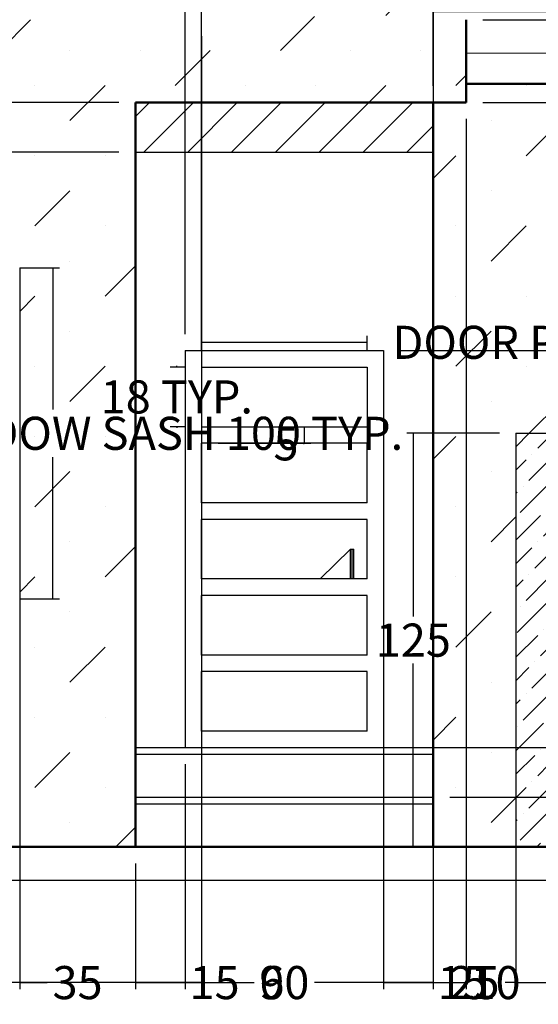
# Model space of a CAD drawing. Units: millimetres. Extents: x 301 to 1039, y -12 to 673.
# Tile 2 of 6: x 579 to 736, y -12 to 285. Entities that reach past the tile are written whole.
import ezdxf

# ---------------------------------------------------------------- set-up
doc = ezdxf.new("R2010")
doc.units = ezdxf.units.MM
doc.header["$MEASUREMENT"] = 0
for name, color, linetype, lineweight in [('A-ANNO-DIMS', 2, 'Continuous', 18), ('A-DOOR', 4, 'Continuous', 25), ('A-ELEV', 8, 'Continuous', 25), ('A-FLOR-STRS', 3, 'Continuous', 25), ('A-WALL', 7, 'Continuous', 50), ('A-WALL-PATT', 9, 'Continuous', 13)]:
    doc.layers.add(name, color=color, linetype=linetype, lineweight=lineweight)
doc.styles.get("Standard").update_dxf_attribs({"font": 'arial.ttf'})
doc.dimstyles.get("Standard").update_dxf_attribs({"dimtxt": 10, "dimasz": 0.18, "dimexe": 2, "dimexo": 5, "dimgap": 2, "dimtad": 0, "dimtih": 1, "dimtoh": 1, "dimdec": 0, "dimzin": 0, "dimdsep": 46, "dimtxsty": 'Standard', "dimcen": 0.09, "dimadec": 0, "dimazin": 0, "dimtfac": 1, "dimtdec": 0, "dimtofl": 0, "dimtmove": 0, "dimatfit": 3, "dimfxl": 1, "dimtolj": 1, "dimtzin": 0, "dimarcsym": 0})

# ---------------------------------------------------------------- blocks, each defined once
blk = doc.blocks.new('DOOR-PANEL')
for p, q in [((0, 18), (50, 18)), ((0, 18), (0, 0)), ((50, 18), (50, 0)), ((0, 0), (50, 0))]:
    blk.add_line(p, q)
blk = doc.blocks.new('*D10')
at = {"layer": 'A-ANNO-DIMS', "color": 0, "lineweight": -2, "transparency": 16777216}
for p, q in [((633.79, 185.09), (633.79, 189.59)), ((633.97, 187.59), (683.61, 187.59)), ((683.79, 185.09), (683.79, 189.59)), ((683.79, 187.59), (683.97, 187.59))]:
    blk.add_line(p, q, dxfattribs=at)
at = {"layer": 'A-ANNO-DIMS', "color": 0, "transparency": 16777216}
for points in [[(633.97, 187.62), (633.97, 187.56), (633.79, 187.59)], [(683.61, 187.62), (683.61, 187.56), (683.79, 187.59)]]:
    blk.add_solid(points, dxfattribs=at)
at = {"layer": 'Defpoints', "color": 0, "transparency": 16777216}
for p in [(683.79, 187.59), (633.79, 180.09), (683.79, 180.09)]:
    blk.add_point(p, dxfattribs=at)
at = {"layer": 'A-ANNO-DIMS', "color": 0, "transparency": 16777216, "insert": (757.8, 187.59), "char_height": 10, "attachment_point": 5}
blk.add_mtext('\\A1;DOOR PANEL 50 TYP.', dxfattribs=at)
blk = doc.blocks.new('*D11')
at = {"layer": 'A-ANNO-DIMS', "color": 0, "lineweight": -2, "transparency": 16777216}
for p, q in [((628.79, 180.09), (624.29, 180.09)), ((626.29, 180.27), (626.29, 180.45)), ((628.79, 162.09), (624.29, 162.09)), ((626.29, 161.91), (626.29, 161.73))]:
    blk.add_line(p, q, dxfattribs=at)
at = {"layer": 'A-ANNO-DIMS', "color": 0, "transparency": 16777216}
for points in [[(626.26, 180.27), (626.32, 180.27), (626.29, 180.09)], [(626.26, 161.91), (626.32, 161.91), (626.29, 162.09)]]:
    blk.add_solid(points, dxfattribs=at)
at = {"layer": 'Defpoints', "color": 0, "transparency": 16777216}
for p in [(626.29, 180.09), (633.79, 180.09), (633.79, 162.09)]:
    blk.add_point(p, dxfattribs=at)
at = {"layer": 'A-ANNO-DIMS', "color": 0, "transparency": 16777216, "insert": (626.29, 171.09), "char_height": 10, "attachment_point": 5}
blk.add_mtext('\\A1;18 TYP.', dxfattribs=at)
blk = doc.blocks.new('*D14')
at = {"layer": 'A-ANNO-DIMS', "color": 0, "lineweight": -2, "transparency": 16777216}
for p, q in [((578.79, 210.09), (590.79, 210.09)), ((588.79, 209.91), (588.79, 167.26)), ((588.79, 110.27), (588.79, 152.91)), ((578.79, 110.09), (590.79, 110.09))]:
    blk.add_line(p, q, dxfattribs=at)
at = {"layer": 'A-ANNO-DIMS', "color": 0, "transparency": 16777216}
for points in [[(588.76, 209.91), (588.82, 209.91), (588.79, 210.09)], [(588.76, 110.27), (588.82, 110.27), (588.79, 110.09)]]:
    blk.add_solid(points, dxfattribs=at)
at = {"layer": 'Defpoints', "color": 0, "transparency": 16777216}
for p in [(573.79, 210.09), (588.79, 210.09), (573.79, 110.09)]:
    blk.add_point(p, dxfattribs=at)
at = {"layer": 'A-ANNO-DIMS', "color": 0, "transparency": 16777216, "insert": (588.79, 160.09), "char_height": 10, "attachment_point": 5}
blk.add_mtext('\\A1;GROUND WINDOW SASH 100 TYP.', dxfattribs=at)
blk = doc.blocks.new('*D20')
at = {"layer": 'A-ANNO-DIMS', "color": 0, "lineweight": -2, "transparency": 16777216}
for p, q in [((343.79, 30.09), (343.79, 668.09)), ((953.79, 30.09), (953.79, 668.09)), ((343.97, 666.09), (635.73, 666.09)), ((953.61, 666.09), (661.85, 666.09))]:
    blk.add_line(p, q, dxfattribs=at)
at = {"layer": 'A-ANNO-DIMS', "color": 0, "transparency": 16777216}
for points in [[(343.97, 666.12), (343.97, 666.06), (343.79, 666.09)], [(953.61, 666.12), (953.61, 666.06), (953.79, 666.09)]]:
    blk.add_solid(points, dxfattribs=at)
at = {"layer": 'Defpoints', "color": 0, "transparency": 16777216}
for p in [(953.79, 666.09), (343.79, 25.09), (953.79, 25.09)]:
    blk.add_point(p, dxfattribs=at)
at = {"layer": 'A-ANNO-DIMS', "color": 0, "transparency": 16777216, "insert": (648.79, 666.09), "char_height": 10, "attachment_point": 5}
blk.add_mtext('\\A1;610', dxfattribs=at)
blk = doc.blocks.new('*D24')
at = {"layer": 'A-ANNO-DIMS', "color": 0, "lineweight": -2, "transparency": 16777216}
for p, q in [((578.79, 210.09), (578.79, -7.91)), ((428.79, 100.09), (428.79, -7.91)), ((428.97, -5.91), (491.23, -5.91)), ((578.61, -5.91), (516.35, -5.91))]:
    blk.add_line(p, q, dxfattribs=at)
at = {"layer": 'A-ANNO-DIMS', "color": 0, "transparency": 16777216}
for points in [[(428.97, -5.88), (428.97, -5.94), (428.79, -5.91)], [(578.61, -5.88), (578.61, -5.94), (578.79, -5.91)]]:
    blk.add_solid(points, dxfattribs=at)
at = {"layer": 'Defpoints', "color": 0, "transparency": 16777216}
for p in [(578.79, 215.09), (428.79, 105.09), (578.79, -5.91)]:
    blk.add_point(p, dxfattribs=at)
at = {"layer": 'A-ANNO-DIMS', "color": 0, "transparency": 16777216, "insert": (503.79, -5.91), "char_height": 10, "attachment_point": 5}
blk.add_mtext('\\A1;150', dxfattribs=at)
blk = doc.blocks.new('*D25')
at = {"layer": 'A-ANNO-DIMS', "color": 0, "lineweight": -2, "transparency": 16777216}
for p, q in [((578.79, 100.09), (578.79, -7.91)), ((613.79, 30.09), (613.79, -7.91)), ((578.97, -5.91), (587.09, -5.91)), ((613.61, -5.91), (605.48, -5.91))]:
    blk.add_line(p, q, dxfattribs=at)
at = {"layer": 'A-ANNO-DIMS', "color": 0, "transparency": 16777216}
for points in [[(578.97, -5.88), (578.97, -5.94), (578.79, -5.91)], [(613.61, -5.88), (613.61, -5.94), (613.79, -5.91)]]:
    blk.add_solid(points, dxfattribs=at)
at = {"layer": 'Defpoints', "color": 0, "transparency": 16777216}
for p in [(578.79, 105.09), (613.79, 35.09), (613.79, -5.91)]:
    blk.add_point(p, dxfattribs=at)
at = {"layer": 'A-ANNO-DIMS', "color": 0, "transparency": 16777216, "insert": (596.29, -5.91), "char_height": 10, "attachment_point": 5}
blk.add_mtext('\\A1;35', dxfattribs=at)
blk = doc.blocks.new('*D26')
at = {"layer": 'A-ANNO-DIMS', "color": 0, "lineweight": -2, "transparency": 16777216}
for p, q in [((703.79, 530.09), (703.79, -7.91)), ((613.79, 30.09), (613.79, -7.91)), ((613.97, -5.91), (649.64, -5.91)), ((703.61, -5.91), (667.93, -5.91))]:
    blk.add_line(p, q, dxfattribs=at)
at = {"layer": 'A-ANNO-DIMS', "color": 0, "transparency": 16777216}
for points in [[(613.97, -5.88), (613.97, -5.94), (613.79, -5.91)], [(703.61, -5.88), (703.61, -5.94), (703.79, -5.91)]]:
    blk.add_solid(points, dxfattribs=at)
at = {"layer": 'Defpoints', "color": 0, "transparency": 16777216}
for p in [(703.79, 535.09), (613.79, 35.09), (703.79, -5.91)]:
    blk.add_point(p, dxfattribs=at)
at = {"layer": 'A-ANNO-DIMS', "color": 0, "transparency": 16777216, "insert": (658.79, -5.91), "char_height": 10, "attachment_point": 5}
blk.add_mtext('\\A1;90', dxfattribs=at)
blk = doc.blocks.new('*D27')
at = {"layer": 'A-ANNO-DIMS', "color": 0, "lineweight": -2, "transparency": 16777216}
for p, q in [((703.79, 530.09), (703.79, -7.91)), ((728.79, 155.09), (728.79, -7.91)), ((703.97, -5.91), (707, -5.91)), ((728.61, -5.91), (725.57, -5.91))]:
    blk.add_line(p, q, dxfattribs=at)
at = {"layer": 'A-ANNO-DIMS', "color": 0, "transparency": 16777216}
for points in [[(703.97, -5.88), (703.97, -5.94), (703.79, -5.91)], [(728.61, -5.88), (728.61, -5.94), (728.79, -5.91)]]:
    blk.add_solid(points, dxfattribs=at)
at = {"layer": 'Defpoints', "color": 0, "transparency": 16777216}
for p in [(703.79, 535.09), (728.79, 160.09), (728.79, -5.91)]:
    blk.add_point(p, dxfattribs=at)
at = {"layer": 'A-ANNO-DIMS', "color": 0, "transparency": 16777216, "insert": (716.29, -5.91), "char_height": 10, "attachment_point": 5}
blk.add_mtext('\\A1;25', dxfattribs=at)
blk = doc.blocks.new('*D28')
at = {"layer": 'A-ANNO-DIMS', "color": 0, "lineweight": -2, "transparency": 16777216}
for p, q in [((728.79, 155.09), (728.79, -7.91)), ((878.79, 155.09), (878.79, -7.91)), ((728.97, -5.91), (791.23, -5.91)), ((878.61, -5.91), (816.35, -5.91))]:
    blk.add_line(p, q, dxfattribs=at)
at = {"layer": 'A-ANNO-DIMS', "color": 0, "transparency": 16777216}
for points in [[(728.97, -5.88), (728.97, -5.94), (728.79, -5.91)], [(878.61, -5.88), (878.61, -5.94), (878.79, -5.91)]]:
    blk.add_solid(points, dxfattribs=at)
at = {"layer": 'Defpoints', "color": 0, "transparency": 16777216}
for p in [(728.79, 160.09), (878.79, 160.09), (878.79, -5.91)]:
    blk.add_point(p, dxfattribs=at)
at = {"layer": 'A-ANNO-DIMS', "color": 0, "transparency": 16777216, "insert": (803.79, -5.91), "char_height": 10, "attachment_point": 5}
blk.add_mtext('\\A1;150', dxfattribs=at)
blk = doc.blocks.new('*D40')
at = {"layer": 'A-ANNO-DIMS', "color": 0, "lineweight": -2, "transparency": 16777216}
for p, q in [((723.79, 160.09), (695.79, 160.09)), ((697.79, 159.91), (697.79, 104.69)), ((697.79, 35.27), (697.79, 90.48)), ((723.79, 35.09), (695.79, 35.09))]:
    blk.add_line(p, q, dxfattribs=at)
at = {"layer": 'A-ANNO-DIMS', "color": 0, "transparency": 16777216}
for points in [[(697.76, 159.91), (697.82, 159.91), (697.79, 160.09)], [(697.76, 35.27), (697.82, 35.27), (697.79, 35.09)]]:
    blk.add_solid(points, dxfattribs=at)
at = {"layer": 'Defpoints', "color": 0, "transparency": 16777216}
for p in [(697.79, 160.09), (728.79, 160.09), (728.79, 35.09)]:
    blk.add_point(p, dxfattribs=at)
at = {"layer": 'A-ANNO-DIMS', "color": 0, "transparency": 16777216, "insert": (697.79, 97.59), "char_height": 10, "attachment_point": 5}
blk.add_mtext('\\A1;125', dxfattribs=at)
blk = doc.blocks.new('*D51')
at = {"layer": 'A-ANNO-DIMS', "color": 0, "lineweight": -2, "transparency": 16777216}
for p, q in [((448.79, 280.09), (448.79, -7.91)), ((633.79, 280.09), (633.79, -7.91)), ((448.97, -5.91), (528.67, -5.91)), ((633.61, -5.91), (553.9, -5.91))]:
    blk.add_line(p, q, dxfattribs=at)
at = {"layer": 'A-ANNO-DIMS', "color": 0, "transparency": 16777216}
for points in [[(448.97, -5.88), (448.97, -5.94), (448.79, -5.91)], [(633.61, -5.88), (633.61, -5.94), (633.79, -5.91)]]:
    blk.add_solid(points, dxfattribs=at)
at = {"layer": 'Defpoints', "color": 0, "transparency": 16777216}
for p in [(448.79, 285.09), (633.79, 285.09), (633.79, -5.91)]:
    blk.add_point(p, dxfattribs=at)
at = {"layer": 'A-ANNO-DIMS', "color": 0, "transparency": 16777216, "insert": (541.29, -5.91), "char_height": 10, "attachment_point": 5}
blk.add_mtext('\\A1;185', dxfattribs=at)
blk = doc.blocks.new('*D52')
at = {"layer": 'A-ANNO-DIMS', "color": 0, "lineweight": -2, "transparency": 16777216}
for p, q in [((666.29, 402.33), (666.29, 668.09)), ((703.79, 265.09), (703.79, 668.09)), ((666.47, 666.09), (670.02, 666.09)), ((703.61, 666.09), (700.06, 666.09))]:
    blk.add_line(p, q, dxfattribs=at)
at = {"layer": 'A-ANNO-DIMS', "color": 0, "transparency": 16777216}
for points in [[(666.47, 666.12), (666.47, 666.06), (666.29, 666.09)], [(703.61, 666.12), (703.61, 666.06), (703.79, 666.09)]]:
    blk.add_solid(points, dxfattribs=at)
at = {"layer": 'Defpoints', "color": 0, "transparency": 16777216}
for p in [(703.79, 666.09), (666.29, 397.33), (703.79, 260.09)]:
    blk.add_point(p, dxfattribs=at)
at = {"layer": 'A-ANNO-DIMS', "color": 0, "transparency": 16777216, "insert": (685.04, 666.09), "char_height": 10, "attachment_point": 5}
blk.add_mtext('\\A1;37.5', dxfattribs=at)
blk = doc.blocks.new('*D53')
at = {"layer": 'A-ANNO-DIMS', "color": 0, "lineweight": -2, "transparency": 16777216}
for p, q in [((703.79, 255.09), (703.79, -7.91)), ((713.79, 255.09), (713.79, -7.91)), ((703.97, -5.91), (713.61, -5.91)), ((713.79, -5.91), (713.97, -5.91))]:
    blk.add_line(p, q, dxfattribs=at)
at = {"layer": 'A-ANNO-DIMS', "color": 0, "transparency": 16777216}
for points in [[(703.97, -5.88), (703.97, -5.94), (703.79, -5.91)], [(713.61, -5.88), (713.61, -5.94), (713.79, -5.91)]]:
    blk.add_solid(points, dxfattribs=at)
at = {"layer": 'Defpoints', "color": 0, "transparency": 16777216}
for p in [(703.79, 260.09), (713.79, 260.09), (713.79, -5.91)]:
    blk.add_point(p, dxfattribs=at)
at = {"layer": 'A-ANNO-DIMS', "color": 0, "transparency": 16777216, "insert": (722.64, -5.91), "char_height": 10, "attachment_point": 5}
blk.add_mtext('\\A1;10', dxfattribs=at)
blk = doc.blocks.new('*D55')
at = {"layer": 'A-ANNO-DIMS', "color": 0, "lineweight": -2, "transparency": 16777216}
for p, q in [((718.79, 285.09), (986.79, 285.09)), ((984.79, 284.91), (984.79, 279.69)), ((984.79, 260.27), (984.79, 265.48)), ((718.79, 260.09), (986.79, 260.09))]:
    blk.add_line(p, q, dxfattribs=at)
at = {"layer": 'A-ANNO-DIMS', "color": 0, "transparency": 16777216}
for points in [[(984.76, 284.91), (984.82, 284.91), (984.79, 285.09)], [(984.76, 260.27), (984.82, 260.27), (984.79, 260.09)]]:
    blk.add_solid(points, dxfattribs=at)
at = {"layer": 'Defpoints', "color": 0, "transparency": 16777216}
for p in [(713.79, 285.09), (984.79, 285.09), (713.79, 260.09)]:
    blk.add_point(p, dxfattribs=at)
at = {"layer": 'A-ANNO-DIMS', "color": 0, "transparency": 16777216, "insert": (984.79, 272.59), "char_height": 10, "attachment_point": 5}
blk.add_mtext('\\A1;25', dxfattribs=at)
blk = doc.blocks.new('*D56')
at = {"layer": 'A-ANNO-DIMS', "color": 0, "lineweight": -2, "transparency": 16777216}
for p, q in [((718.79, 335.09), (986.79, 335.09)), ((984.79, 334.91), (984.79, 317.19)), ((984.79, 285.27), (984.79, 302.98)), ((718.79, 285.09), (986.79, 285.09))]:
    blk.add_line(p, q, dxfattribs=at)
at = {"layer": 'A-ANNO-DIMS', "color": 0, "transparency": 16777216}
for points in [[(984.76, 334.91), (984.82, 334.91), (984.79, 335.09)], [(984.76, 285.27), (984.82, 285.27), (984.79, 285.09)]]:
    blk.add_solid(points, dxfattribs=at)
at = {"layer": 'Defpoints', "color": 0, "transparency": 16777216}
for p in [(713.79, 335.09), (984.79, 335.09), (713.79, 285.09)]:
    blk.add_point(p, dxfattribs=at)
at = {"layer": 'A-ANNO-DIMS', "color": 0, "transparency": 16777216, "insert": (984.79, 310.09), "char_height": 10, "attachment_point": 5}
blk.add_mtext('\\A1;50', dxfattribs=at)
blk = doc.blocks.new('*D64')
at = {"layer": 'A-ANNO-DIMS', "color": 0, "lineweight": -2, "transparency": 16777216}
for p, q in [((608.79, 245.09), (310.79, 245.09)), ((312.79, 244.91), (312.79, 147.19)), ((312.79, 35.27), (312.79, 132.98)), ((608.79, 35.09), (310.79, 35.09))]:
    blk.add_line(p, q, dxfattribs=at)
at = {"layer": 'A-ANNO-DIMS', "color": 0, "transparency": 16777216}
for points in [[(312.76, 244.91), (312.82, 244.91), (312.79, 245.09)], [(312.76, 35.27), (312.82, 35.27), (312.79, 35.09)]]:
    blk.add_solid(points, dxfattribs=at)
at = {"layer": 'Defpoints', "color": 0, "transparency": 16777216}
for p in [(312.79, 245.09), (613.79, 245.09), (613.79, 35.09)]:
    blk.add_point(p, dxfattribs=at)
at = {"layer": 'A-ANNO-DIMS', "color": 0, "transparency": 16777216, "insert": (312.79, 140.09), "char_height": 10, "attachment_point": 5}
blk.add_mtext('\\A1;210', dxfattribs=at)
blk = doc.blocks.new('*D65')
at = {"layer": 'A-ANNO-DIMS', "color": 0, "lineweight": -2, "transparency": 16777216}
for p, q in [((608.788413, 260.088152), (310.788413, 260.088152)), ((312.788413, 260.268152), (312.788413, 260.448152)), ((608.788413, 245.088152), (310.788413, 245.088152)), ((312.788413, 244.908152), (312.788413, 244.728152))]:
    blk.add_line(p, q, dxfattribs=at)
at = {"layer": 'A-ANNO-DIMS', "color": 0, "transparency": 16777216}
for points in [[(312.758413, 260.268152), (312.818413, 260.268152), (312.788413, 260.088152)], [(312.758413, 244.908152), (312.818413, 244.908152), (312.788413, 245.088152)]]:
    blk.add_solid(points, dxfattribs=at)
at = {"layer": 'Defpoints', "color": 0, "transparency": 16777216}
for p in [(312.788413, 260.088152), (613.788413, 260.088152), (613.788413, 245.088152)]:
    blk.add_point(p, dxfattribs=at)
at = {"layer": 'A-ANNO-DIMS', "color": 0, "transparency": 16777216, "insert": (312.788413, 252.588152), "char_height": 10, "attachment_point": 5}
blk.add_mtext('\\A1;15', dxfattribs=at)
blk = doc.blocks.new('*D66')
at = {"layer": 'A-ANNO-DIMS', "color": 0, "lineweight": -2, "transparency": 16777216}
for p, q in [((628.79, 60.09), (628.79, -7.91)), ((613.79, 30.09), (613.79, -7.91)), ((613.97, -5.91), (628.61, -5.91)), ((628.79, -5.91), (628.97, -5.91))]:
    blk.add_line(p, q, dxfattribs=at)
at = {"layer": 'A-ANNO-DIMS', "color": 0, "transparency": 16777216}
for points in [[(613.97, -5.88), (613.97, -5.94), (613.79, -5.91)], [(628.61, -5.88), (628.61, -5.94), (628.79, -5.91)]]:
    blk.add_solid(points, dxfattribs=at)
at = {"layer": 'Defpoints', "color": 0, "transparency": 16777216}
for p in [(628.79, 65.09), (613.79, 35.09), (628.79, -5.91)]:
    blk.add_point(p, dxfattribs=at)
at = {"layer": 'A-ANNO-DIMS', "color": 0, "transparency": 16777216, "insert": (637.7, -5.91), "char_height": 10, "attachment_point": 5}
blk.add_mtext('\\A1;15', dxfattribs=at)
blk = doc.blocks.new('*D67')
at = {"layer": 'A-ANNO-DIMS', "color": 0, "lineweight": -2, "transparency": 16777216}
for p, q in [((688.79, 180.09), (688.79, -7.91)), ((628.79, 60.09), (628.79, -7.91)), ((628.97, -5.91), (649.62, -5.91)), ((688.61, -5.91), (667.96, -5.91))]:
    blk.add_line(p, q, dxfattribs=at)
at = {"layer": 'A-ANNO-DIMS', "color": 0, "transparency": 16777216}
for points in [[(628.97, -5.88), (628.97, -5.94), (628.79, -5.91)], [(688.61, -5.88), (688.61, -5.94), (688.79, -5.91)]]:
    blk.add_solid(points, dxfattribs=at)
at = {"layer": 'Defpoints', "color": 0, "transparency": 16777216}
for p in [(688.79, 185.09), (628.79, 65.09), (688.79, -5.91)]:
    blk.add_point(p, dxfattribs=at)
at = {"layer": 'A-ANNO-DIMS', "color": 0, "transparency": 16777216, "insert": (658.79, -5.91), "char_height": 10, "attachment_point": 5}
blk.add_mtext('\\A1;60', dxfattribs=at)
blk = doc.blocks.new('*D68')
at = {"layer": 'A-ANNO-DIMS', "color": 0, "lineweight": -2, "transparency": 16777216}
for p, q in [((688.79, 60.09), (688.79, -7.91)), ((703.79, 60.09), (703.79, -7.91)), ((688.97, -5.91), (703.61, -5.91)), ((703.79, -5.91), (703.97, -5.91))]:
    blk.add_line(p, q, dxfattribs=at)
at = {"layer": 'A-ANNO-DIMS', "color": 0, "transparency": 16777216}
for points in [[(688.97, -5.88), (688.97, -5.94), (688.79, -5.91)], [(703.61, -5.88), (703.61, -5.94), (703.79, -5.91)]]:
    blk.add_solid(points, dxfattribs=at)
at = {"layer": 'Defpoints', "color": 0, "transparency": 16777216}
for p in [(688.79, 65.09), (703.79, 65.09), (703.79, -5.91)]:
    blk.add_point(p, dxfattribs=at)
at = {"layer": 'A-ANNO-DIMS', "color": 0, "transparency": 16777216, "insert": (712.7, -5.91), "char_height": 10, "attachment_point": 5}
blk.add_mtext('\\A1;15', dxfattribs=at)
blk = doc.blocks.new('*D69')
at = {"layer": 'A-ANNO-DIMS', "color": 0, "lineweight": -2, "transparency": 16777216}
for p, q in [((708.788413, 50.088152), (986.788413, 50.088152)), ((984.788413, 50.268152), (984.788413, 50.448152)), ((708.788413, 35.088152), (986.788413, 35.088152)), ((984.788413, 34.908152), (984.788413, 34.728152))]:
    blk.add_line(p, q, dxfattribs=at)
at = {"layer": 'A-ANNO-DIMS', "color": 0, "transparency": 16777216}
for points in [[(984.758413, 50.268152), (984.818413, 50.268152), (984.788413, 50.088152)], [(984.758413, 34.908152), (984.818413, 34.908152), (984.788413, 35.088152)]]:
    blk.add_solid(points, dxfattribs=at)
at = {"layer": 'Defpoints', "color": 0, "transparency": 16777216}
for p in [(703.788413, 50.088152), (984.788413, 50.088152), (703.788413, 35.088152)]:
    blk.add_point(p, dxfattribs=at)
at = {"layer": 'A-ANNO-DIMS', "color": 0, "transparency": 16777216, "insert": (984.788413, 42.588152), "char_height": 10, "attachment_point": 5}
blk.add_mtext('\\A1;15', dxfattribs=at)
blk = doc.blocks.new('*D70')
at = {"layer": 'A-ANNO-DIMS', "color": 0, "lineweight": -2, "transparency": 16777216}
for p, q in [((708.788413, 65.088152), (986.788413, 65.088152)), ((984.788413, 65.268152), (984.788413, 65.448152)), ((708.788413, 50.088152), (986.788413, 50.088152)), ((984.788413, 49.908152), (984.788413, 49.728152))]:
    blk.add_line(p, q, dxfattribs=at)
at = {"layer": 'A-ANNO-DIMS', "color": 0, "transparency": 16777216}
for points in [[(984.758413, 65.268152), (984.818413, 65.268152), (984.788413, 65.088152)], [(984.758413, 49.908152), (984.818413, 49.908152), (984.788413, 50.088152)]]:
    blk.add_solid(points, dxfattribs=at)
at = {"layer": 'Defpoints', "color": 0, "transparency": 16777216}
for p in [(703.788413, 65.088152), (984.788413, 65.088152), (703.788413, 50.088152)]:
    blk.add_point(p, dxfattribs=at)
at = {"layer": 'A-ANNO-DIMS', "color": 0, "transparency": 16777216, "insert": (984.788413, 57.588152), "char_height": 10, "attachment_point": 5}
blk.add_mtext('\\A1;15', dxfattribs=at)
blk = doc.blocks.new('*D71')
at = {"layer": 'A-ANNO-DIMS', "color": 0, "lineweight": -2, "transparency": 16777216}
for p, q in [((693.79, 185.09), (986.79, 185.09)), ((984.79, 184.91), (984.79, 132.19)), ((984.79, 65.27), (984.79, 117.98)), ((693.79, 65.09), (986.79, 65.09))]:
    blk.add_line(p, q, dxfattribs=at)
at = {"layer": 'A-ANNO-DIMS', "color": 0, "transparency": 16777216}
for points in [[(984.76, 184.91), (984.82, 184.91), (984.79, 185.09)], [(984.76, 65.27), (984.82, 65.27), (984.79, 65.09)]]:
    blk.add_solid(points, dxfattribs=at)
at = {"layer": 'Defpoints', "color": 0, "transparency": 16777216}
for p in [(688.79, 185.09), (984.79, 185.09), (688.79, 65.09)]:
    blk.add_point(p, dxfattribs=at)
at = {"layer": 'A-ANNO-DIMS', "color": 0, "transparency": 16777216, "insert": (984.79, 125.09), "char_height": 10, "attachment_point": 5}
blk.add_mtext('\\A1;120', dxfattribs=at)
blk = doc.blocks.new('*D72')
at = {"layer": 'A-ANNO-DIMS', "color": 0, "lineweight": -2, "transparency": 16777216}
for p, q in [((628.79, 190.09), (628.79, 668.09)), ((633.79, 185.09), (633.79, 668.09)), ((628.97, 666.09), (633.61, 666.09)), ((633.79, 666.09), (633.97, 666.09))]:
    blk.add_line(p, q, dxfattribs=at)
at = {"layer": 'A-ANNO-DIMS', "color": 0, "transparency": 16777216}
for points in [[(628.97, 666.12), (628.97, 666.06), (628.79, 666.09)], [(633.61, 666.12), (633.61, 666.06), (633.79, 666.09)]]:
    blk.add_solid(points, dxfattribs=at)
at = {"layer": 'Defpoints', "color": 0, "transparency": 16777216}
for p in [(633.79, 666.09), (628.79, 185.09), (633.79, 180.09)]:
    blk.add_point(p, dxfattribs=at)
at = {"layer": 'A-ANNO-DIMS', "color": 0, "transparency": 16777216, "insert": (639.28, 666.09), "char_height": 10, "attachment_point": 5}
blk.add_mtext('\\A1;5', dxfattribs=at)
blk = doc.blocks.new('*D73')
at = {"layer": 'A-ANNO-DIMS', "color": 0, "lineweight": -2, "transparency": 16777216}
for p, q in [((638.79, 162.09), (666.79, 162.09)), ((664.79, 161.91), (664.79, 157.27)), ((638.79, 157.09), (666.79, 157.09)), ((664.79, 156.91), (664.61, 156.91)), ((664.79, 157.09), (664.79, 156.91))]:
    blk.add_line(p, q, dxfattribs=at)
at = {"layer": 'A-ANNO-DIMS', "color": 0, "transparency": 16777216}
for points in [[(664.76, 161.91), (664.82, 161.91), (664.79, 162.09)], [(664.76, 157.27), (664.82, 157.27), (664.79, 157.09)]]:
    blk.add_solid(points, dxfattribs=at)
at = {"layer": 'Defpoints', "color": 0, "transparency": 16777216}
for p in [(633.79, 162.09), (633.79, 157.09), (664.79, 157.09)]:
    blk.add_point(p, dxfattribs=at)
at = {"layer": 'A-ANNO-DIMS', "color": 0, "transparency": 16777216, "insert": (659.29, 156.91), "char_height": 10, "attachment_point": 5}
blk.add_mtext('\\A1;5', dxfattribs=at)

msp = doc.modelspace()

# ---------------------------------------------------------------- hatches: boundary and pattern name
at = {"layer": 'A-WALL-PATT'}
h = msp.add_hatch(dxfattribs=at)
h.set_pattern_fill('ANSI31', color=256, scale=100, angle=135)
h.paths.add_polyline_path([(903.788, 585.088), (703.788, 585.088), (703.788, 535.088), (723.788, 535.088), (723.788, 505.088), (703.788, 505.088), (703.788, 335.088), (713.788, 335.088), (713.788, 333.088), (703.788, 333.088), (703.788, 285.088), (713.788, 285.088), (713.788, 265.672), (903.788, 265.672)])
h.paths.add_polyline_path([(868.687, 420.264), (868.687, 290.264), (738.687, 290.264), (738.687, 420.264)], flags=16)
h.paths.add_polyline_path([(866.687, 418.264), (866.687, 292.264), (740.687, 292.264), (740.687, 418.264)], flags=0)
h.paths.add_polyline_path([(861.687, 413.264), (861.687, 297.264), (745.687, 297.264), (745.687, 413.264)], flags=0)
h.paths.add_polyline_path([(860.687, 412.264), (860.687, 298.264), (809.687, 298.264), (809.687, 412.264)], flags=0)
h.paths.add_polyline_path([(797.687, 412.264), (797.687, 298.264), (746.687, 298.264), (746.687, 412.264)], flags=0)
h = msp.add_hatch(dxfattribs=at)
h.set_pattern_fill('MUDST', color=256, scale=60, angle=45)
edge = h.paths.add_edge_path()
edge.add_line((703.788, 505.088), (403.788, 505.088))
edge.add_line((403.788, 505.088), (403.788, 335.088))
edge.add_line((403.788, 335.088), (448.788, 335.088))
edge.add_line((448.788, 335.088), (448.788, 400.52))
edge.add_line((448.788, 400.52), (448.788, 440.088))
edge.add_line((448.788, 440.088), (633.788, 440.088))
edge.add_line((633.788, 440.088), (633.788, 400.52))
edge.add_line((633.788, 400.52), (633.788, 335.088))
edge.add_line((633.788, 335.088), (673.88, 335.088))
edge.add_spline(control_points=[(673.88, 335.088), (673.929, 335.734), (674.283, 339.462), (675.587, 346.794), (678.602, 339.909), (679.226, 336.718), (679.369, 335.088)], knot_values=[26.7052686, 26.7052686, 26.7052686, 26.7052686, 28.3156814, 35.5227919, 39.6456178, 44.5318346, 44.5318346, 44.5318346, 44.5318346], degree=3, periodic=0)
edge.add_line((679.369, 335.088), (703.788, 335.088))
edge.add_line((703.788, 335.088), (703.788, 505.088))
h.paths.add_polyline_path([(681.292, 397.334, -1), (651.292, 397.334, -1)], flags=16)
h.paths.add_polyline_path([(679.292, 397.334, -1), (653.292, 397.334, -1)], flags=0)
h.paths.add_polyline_path([(448.788, 333.088), (403.788, 333.088), (403.788, 285.088), (448.788, 285.088)])
h.paths.add_polyline_path([(613.788, 260.088), (713.788, 260.088), (713.788, 285.088), (403.788, 285.088), (393.788, 285.088), (393.788, 35.088), (403.788, 35.088), (613.788, 35.088)])
h.paths.add_polyline_path([(578.788, 215.088), (578.788, 105.088), (428.788, 105.088), (428.788, 215.088)], flags=16)
h.paths.add_polyline_path([(501.288, 210.088), (501.288, 185.088), (433.788, 185.088), (433.788, 210.088)], flags=0)
h.paths.add_polyline_path([(501.288, 180.088), (501.288, 110.088), (433.788, 110.088), (433.788, 180.088)], flags=0)
h.paths.add_polyline_path([(506.288, 210.088), (573.788, 210.088), (573.788, 185.088), (506.288, 185.088)], flags=0)
h.paths.add_polyline_path([(506.288, 180.088), (573.788, 180.088), (573.788, 110.088), (506.288, 110.088)], flags=0)
edge = h.paths.add_edge_path()
edge.add_spline(control_points=[(675.148, 309.006), (675.282, 309.92), (671.965, 311.304), (670.019, 313.17), (668.379, 316.485), (667.076, 320.028), (669.149, 324.142), (672.687, 322.877), (673.644, 321.553), (673.786, 321.296)], knot_values=[12.4980994, 12.4980994, 12.4980994, 12.4980994, 15.7345293, 18.1242776, 22.0598536, 26.1694355, 29.2709867, 33.3603853, 34.273637, 34.273637, 34.273637, 34.273637], degree=3, periodic=0)
edge.add_spline(control_points=[(673.786, 321.296), (673.373, 322.666), (672.565, 324.662), (673.805, 325.84), (674.246, 326.099)], knot_values=[12.3304253, 12.3304253, 12.3304253, 12.3304253, 16.1943692, 17.6683934, 17.6683934, 17.6683934, 17.6683934], degree=3, periodic=0)
edge.add_spline(control_points=[(674.246, 326.099), (673.92, 328.298), (673.697, 330.39), (673.774, 333.088)], knot_values=[46.2924512, 46.2924512, 46.2924512, 46.2924512, 53.8278009, 53.8278009, 53.8278009, 53.8278009], degree=3, periodic=0)
edge.add_line((673.774, 333.088), (648.788, 333.088))
edge.add_line((648.788, 333.088), (648.788, 285.088))
edge.add_line((648.788, 285.088), (666.788, 285.088))
edge.add_line((666.788, 285.088), (664.215, 309.96))
edge.add_arc((676.288, 385.148), 76.15, 260.87778, 269.14183)
edge = h.paths.add_edge_path()
edge.add_line((703.788, 333.088), (679.453, 333.088))
edge.add_spline(control_points=[(679.453, 333.088), (679.452, 331.277), (679.21, 329.205), (678.936, 327.067), (678.889, 326.706)], knot_values=[17.8386285, 17.8386285, 17.8386285, 17.8386285, 23.5111371, 24.6594022, 24.6594022, 24.6594022, 24.6594022], degree=3, periodic=0)
edge.add_spline(control_points=[(678.889, 326.706), (678.729, 326.741), (678.565, 326.771), (678.396, 326.794)], knot_values=[21.2892091, 21.2892091, 21.2892091, 21.2892091, 21.7264211, 21.7264211, 21.7264211, 21.7264211], degree=3, periodic=0)
edge.add_spline(control_points=[(678.396, 326.794), (678.233, 326.816), (678.067, 326.832), (677.898, 326.842)], knot_values=[20.8675669, 20.8675669, 20.8675669, 20.8675669, 21.2892091, 21.2892091, 21.2892091, 21.2892091], degree=3, periodic=0)
edge.add_spline(control_points=[(677.898, 326.842), (676.995, 326.898), (676.024, 326.786), (675.195, 326.517)], knot_values=[18.611077, 18.611077, 18.611077, 18.611077, 20.8675669, 20.8675669, 20.8675669, 20.8675669], degree=3, periodic=0)
edge.add_spline(control_points=[(675.195, 326.517), (675.029, 326.464), (674.869, 326.404), (674.716, 326.337)], knot_values=[18.1593829, 18.1593829, 18.1593829, 18.1593829, 18.611077, 18.611077, 18.611077, 18.611077], degree=3, periodic=0)
edge.add_spline(control_points=[(674.716, 326.337), (674.55, 326.265), (674.392, 326.186), (674.246, 326.099)], knot_values=[17.6683934, 17.6683934, 17.6683934, 17.6683934, 18.1593829, 18.1593829, 18.1593829, 18.1593829], degree=3, periodic=0)
edge.add_spline(control_points=[(674.246, 326.099), (673.805, 325.84), (672.565, 324.662), (673.373, 322.666), (673.786, 321.296)], knot_values=[12.3304253, 12.3304253, 12.3304253, 12.3304253, 13.8044495, 17.6683934, 17.6683934, 17.6683934, 17.6683934], degree=3, periodic=0)
edge.add_spline(control_points=[(673.786, 321.296), (674.162, 320.613), (674.301, 319.823), (674.341, 318.987)], knot_values=[10.0649388, 10.0649388, 10.0649388, 10.0649388, 12.4980994, 12.4980994, 12.4980994, 12.4980994], degree=3, periodic=0)
edge.add_spline(control_points=[(674.341, 318.987), (674.206, 319.737), (674.024, 320.504), (673.786, 321.296)], knot_values=[10.094462, 10.094462, 10.094462, 10.094462, 12.3304253, 12.3304253, 12.3304253, 12.3304253], degree=3, periodic=0)
edge.add_spline(control_points=[(673.786, 321.296), (673.644, 321.553), (672.687, 322.877), (669.149, 324.142), (667.076, 320.028), (668.379, 316.485), (670.019, 313.17), (671.965, 311.304), (675.282, 309.92), (675.148, 309.006)], knot_values=[12.4980994, 12.4980994, 12.4980994, 12.4980994, 13.4113511, 17.5007497, 20.6023009, 24.7118828, 28.6474588, 31.0372071, 34.273637, 34.273637, 34.273637, 34.273637], degree=3, periodic=0)
edge.add_arc((676.288, 385.148), 76.15, 260.87778, 269.14183, ccw=False)
edge.add_line((664.215, 309.96), (666.788, 285.088))
edge.add_line((666.788, 285.088), (703.788, 285.088))
edge.add_line((703.788, 285.088), (703.788, 333.088))
h.paths.add_polyline_path([(687.234, 308.777), (684.887, 286.088), (667.69, 286.088), (665.343, 308.777, 0.0712952)], flags=16)
h.paths.add_polyline_path([(903.788, 265.672), (713.788, 265.672), (713.788, 260.088), (703.788, 260.088), (703.788, 35.088), (728.788, 35.088), (728.788, 160.088), (878.788, 160.088), (878.788, 35.088), (903.788, 35.088)])
h = msp.add_hatch(dxfattribs=at)
h.set_pattern_fill('ANSI31', color=256, scale=75)
h.paths.add_polyline_path([(703.788, 260.088), (613.788, 260.088), (613.788, 245.088), (703.788, 245.088)])
h = msp.add_hatch(dxfattribs=at)
h.set_pattern_fill('ANSI36', color=256, scale=40)
h.paths.add_polyline_path([(878.788, 160.088), (728.788, 160.088), (728.788, 35.088), (738.788, 35.088), (738.788, 150.088), (868.788, 150.088), (868.788, 35.088), (878.788, 35.088)])

# ---------------------------------------------------------------- linework, layer by layer
at = {"layer": 'A-DOOR'}
for p, q in [((628.788, 185.088), (688.788, 185.088)), ((628.788, 185.088), (628.788, 65.088)), ((688.788, 185.088), (688.788, 65.088)), ((728.788, 160.088), (878.788, 160.088)), ((728.788, 160.088), (728.788, 35.088)), ((678.831, 125.11), (669.602, 116.088)), ((678.831, 116.088), (678.831, 125.11)), ((678.831, 125.11), (679.831, 125.11)), ((679.331, 116.088), (679.331, 125.11)), ((679.831, 116.088), (679.831, 125.11))]:
    msp.add_line(p, q, dxfattribs=at)
at = {"layer": 'A-ELEV'}
for p, q in [((613.788, 245.088), (703.788, 245.088)), ((403.788, 25.088), (618.788, 25.088)), ((618.788, 25.088), (953.788, 25.088))]:
    msp.add_line(p, q, dxfattribs=at)
at = {"layer": 'A-FLOR-STRS'}
for p, q in [((613.788, 65.088), (703.788, 65.088)), ((613.788, 63.088), (703.788, 63.088)), ((613.788, 50.088), (703.788, 50.088)), ((613.788, 48.088), (703.788, 48.088))]:
    msp.add_line(p, q, dxfattribs=at)
at = {"layer": 'A-WALL'}
for p, q in [((713.788, 260.088), (713.788, 285.088)), ((713.788, 265.672), (903.788, 265.672)), ((613.788, 260.088), (713.788, 260.088)), ((613.788, 260.088), (613.788, 35.088)), ((703.788, 260.088), (703.788, 35.088)), ((953.788, 35.088), (403.788, 35.088))]:
    msp.add_line(p, q, dxfattribs=at)

# ---------------------------------------------------------------- block references
at = {"layer": 'A-DOOR'}
msp.add_blockref('DOOR-PANEL', (633.788, 162.088), dxfattribs=at)
at = {"layer": 'A-DOOR', "rotation": 180}
for p in [(683.789, 157.088), (683.789, 134.088), (683.789, 111.088), (683.789, 88.088)]:
    msp.add_blockref('DOOR-PANEL', p, dxfattribs=at)

# ---------------------------------------------------------------- dimensions: what is measured, and where the dimension line sits
at = {"layer": 'A-ANNO-DIMS'}
for base, p1, p2, override, picture, middle in [((953.788, 666.088), (343.788, 25.088), (953.788, 25.088), {"dimdec": 0, "dimlfac": 1, "dimrnd": 0, "dimzin": 0, "dimdsep": 46, "dimlunit": 2}, '*D20', (648.788, 666.088)), ((633.788, 666.088), (628.788, 185.088), (633.788, 180.088), {"dimdec": 0, "dimlfac": 1, "dimrnd": 0, "dimzin": 0, "dimdsep": 46, "dimlunit": 2}, '*D72', (639.284, 666.088)), ((703.788, 666.088), (666.292, 397.334), (703.788, 260.088), {"dimdec": 1, "dimlfac": 1, "dimrnd": 0, "dimzin": 0, "dimdsep": 46, "dimlunit": 2}, '*D52', (685.04, 666.088)), ((703.788, -5.912), (613.788, 35.088), (703.788, 535.088), {"dimdec": 0, "dimlfac": 1, "dimrnd": 0, "dimzin": 0, "dimdsep": 46, "dimlunit": 2}, '*D26', (658.788, -5.912)), ((728.788, -5.912), (703.788, 535.088), (728.788, 160.088), {"dimdec": 0, "dimlfac": 1, "dimrnd": 0, "dimzin": 0, "dimdsep": 46, "dimlunit": 2}, '*D27', (716.288, -5.912)), ((633.788, -5.912), (448.788, 285.088), (633.788, 285.088), {"dimdec": 0, "dimlfac": 1, "dimrnd": 0, "dimzin": 0, "dimdsep": 46, "dimlunit": 2}, '*D51', (541.288, -5.912)), ((713.788, -5.912), (703.788, 260.088), (713.788, 260.088), {"dimdec": 0, "dimlfac": 1, "dimrnd": 0, "dimzin": 0, "dimdsep": 46, "dimlunit": 2}, '*D53', (722.643, -5.912)), ((578.788, -5.912), (428.788, 105.088), (578.788, 215.088), {"dimdec": 0, "dimlfac": 1, "dimrnd": 0, "dimzin": 0, "dimdsep": 46, "dimlunit": 2}, '*D24', (503.788, -5.912)), ((688.788, -5.912), (628.788, 65.088), (688.788, 185.088), {"dimdec": 0, "dimlfac": 1, "dimrnd": 0, "dimzin": 0, "dimdsep": 46, "dimlunit": 2}, '*D67', (658.788, -5.912)), ((878.788, -5.912), (728.788, 160.088), (878.788, 160.088), {"dimdec": 0, "dimlfac": 1, "dimrnd": 0, "dimzin": 0, "dimdsep": 46, "dimlunit": 2}, '*D28', (803.788, -5.912)), ((613.788, -5.912), (578.788, 105.088), (613.788, 35.088), {"dimdec": 0, "dimlfac": 1, "dimrnd": 0, "dimzin": 0, "dimdsep": 46, "dimlunit": 2}, '*D25', (596.288, -5.912)), ((628.788, -5.912), (613.788, 35.088), (628.788, 65.088), {"dimdec": 0, "dimlfac": 1, "dimrnd": 0, "dimzin": 0, "dimdsep": 46, "dimlunit": 2}, '*D66', (637.698, -5.912)), ((703.788, -5.912), (688.788, 65.088), (703.788, 65.088), {"dimdec": 0, "dimlfac": 1, "dimrnd": 0, "dimzin": 0, "dimdsep": 46, "dimlunit": 2}, '*D68', (712.698, -5.912))]:
    dim = msp.add_linear_dim(base=base, p1=p1, p2=p2, dimstyle='Standard', override=override, dxfattribs=at)
    dim.commit()
    dim.dimension.update_dxf_attribs({"geometry": picture, "text_midpoint": middle})
for base, p1, p2, angle, picture, middle in [((984.788, 335.088), (713.788, 285.088), (713.788, 335.088), 90, '*D56', (984.788, 310.088)), ((984.788, 285.088), (713.788, 260.088), (713.788, 285.088), 90, '*D55', (984.788, 272.588)), ((312.788, 260.088), (613.788, 245.088), (613.788, 260.088), 90, '*D65', (312.788, 252.588)), ((312.788, 245.088), (613.788, 35.088), (613.788, 245.088), 90, '*D64', (312.788, 140.088)), ((984.788, 185.088), (688.788, 65.088), (688.788, 185.088), 90, '*D71', (984.788, 125.088)), ((664.788, 157.088), (633.788, 162.088), (633.788, 157.088), 270, '*D73', (659.293, 156.908)), ((697.788, 160.088), (728.788, 35.088), (728.788, 160.088), 90, '*D40', (697.788, 97.588)), ((984.788, 65.088), (703.788, 50.088), (703.788, 65.088), 90, '*D70', (984.788, 57.588)), ((984.788, 50.088), (703.788, 35.088), (703.788, 50.088), 90, '*D69', (984.788, 42.588))]:
    dim = msp.add_linear_dim(base=base, p1=p1, p2=p2, angle=angle, dimstyle='Standard', override={"dimdec": 0, "dimlfac": 1, "dimrnd": 0, "dimzin": 0, "dimdsep": 46, "dimlunit": 2}, dxfattribs=at)
    dim.commit()
    dim.dimension.update_dxf_attribs({"geometry": picture, "text_midpoint": middle})
dim = msp.add_linear_dim(base=(683.788, 187.588), p1=(633.788, 180.088), p2=(683.788, 180.088), text='DOOR PANEL <> TYP.', dimstyle='Standard', override={"dimdec": 0, "dimrnd": 0, "dimzin": 0, "dimlunit": 2}, dxfattribs=at)
dim.commit()
dim.dimension.update_dxf_attribs({"geometry": '*D10', "text_midpoint": (757.8, 187.588)})
for base, p1, p2, text, picture, middle in [((588.788, 210.088), (573.788, 110.088), (573.788, 210.088), 'GROUND WINDOW SASH <> TYP.', '*D14', (588.788, 160.088)), ((626.288, 180.088), (633.788, 162.088), (633.788, 180.088), '<> TYP.', '*D11', (626.288, 171.088))]:
    dim = msp.add_linear_dim(base=base, p1=p1, p2=p2, angle=90, text=text, dimstyle='Standard', override={"dimdec": 0, "dimrnd": 0, "dimzin": 0, "dimlunit": 2}, dxfattribs=at)
    dim.commit()
    dim.dimension.update_dxf_attribs({"geometry": picture, "text_midpoint": middle})

doc.saveas('drawing.dxf')
